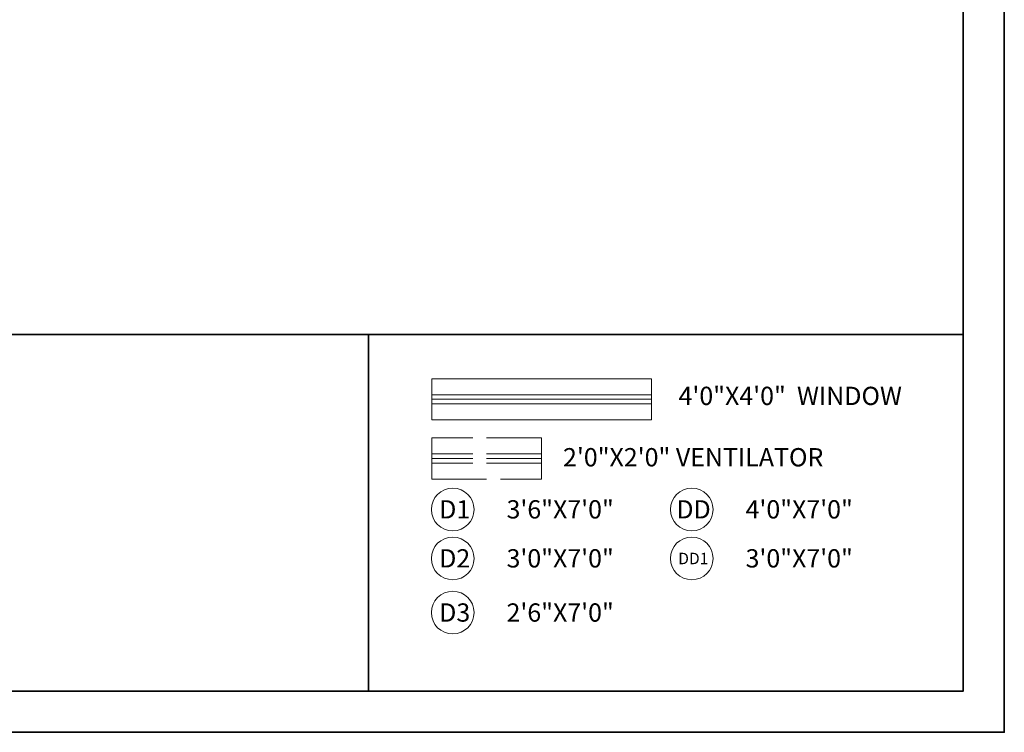
# Model space of a CAD drawing. Units: inches. Extents: x 1077 to 2505, y 1892 to 2728.
# Tile 6 of 26: x 1433 to 1648, y 1892 to 2048. Entities that reach past the tile are written whole.
import ezdxf

# ---------------------------------------------------------------- set-up
doc = ezdxf.new("R2010")
doc.units = ezdxf.units.IN
doc.linetypes.add('ACAD_ISO02W100', pattern=[15, 12, -3])
for name, color, linetype, lineweight in [('A-ANNO-LEGD', 7, 'Continuous', 13), ('A-ANNO-TTLB', 7, 'Continuous', 35), ('A-GLAZ-VENT', 6, 'ACAD_ISO02W100', 13), ('WINDOW', 160, 'Continuous', 13)]:
    doc.layers.add(name, color=color, linetype=linetype, lineweight=lineweight)
doc.styles.get("Standard").update_dxf_attribs({"font": 'arial.ttf'})

# ---------------------------------------------------------------- blocks, each defined once
blk = doc.blocks.new('WINDOW-48-EXT')
for p, q in [((0, 48), (0, 0)), ((3.5, 48), (3.5, 0)), ((4.5, 48), (4.5, 0)), ((5.5, 48), (5.5, 0)), ((9, 0), (9, 48))]:
    blk.add_line(p, q)
blk = doc.blocks.new('VENT-24')
for p, q in [((3.5, 24), (3.5, 0)), ((4.5, 24), (4.5, 0)), ((5.5, 24), (5.5, 0))]:
    blk.add_line(p, q)
blk.add_lwpolyline([(0, 0), (9, 0), (9, 24), (0, 24)], close=True)
blk = doc.blocks.new('SHEET-FRAME-RESIDENTIAL')
for p, q in [((9, 87.01), (534.52, 87.01)), ((404.52, 9), (404.52, 87.01))]:
    blk.add_line(p, q)
for points in [[(0, 830.04), (543.52, 830.04), (543.52, 0), (0, 0)], [(9, 821.04), (534.52, 821.04), (534.52, 9), (9, 9)]]:
    blk.add_lwpolyline(points, close=True)

msp = doc.modelspace()

# ---------------------------------------------------------------- linework, layer by layer
at = {"layer": 'A-ANNO-LEGD'}
for centre in [(1527.2, 1941.03), (1579.45, 1941.03), (1527.2, 1930.32), (1579.45, 1930.32), (1527.2, 1918.46)]:
    msp.add_circle(centre, 4.67, dxfattribs=at)
at = {"layer": 'WINDOW'}
for p, q in [((1522.62, 1969.62), (1522.62, 1960.62)), ((1570.62, 1969.62), (1570.62, 1960.62))]:
    msp.add_line(p, q, dxfattribs=at)

# ---------------------------------------------------------------- block references
at = {"layer": 'A-ANNO-TTLB'}
msp.add_blockref('SHEET-FRAME-RESIDENTIAL', (1104.25, 1892.27), dxfattribs=at)
at = {"layer": 'A-GLAZ-VENT', "rotation": 269.9999999999977}
msp.add_blockref('VENT-24', (1522.62, 1956.67), dxfattribs=at)
at = {"layer": 'WINDOW', "rotation": 89.99999999999969}
msp.add_blockref('WINDOW-48-EXT', (1570.62, 1960.62), dxfattribs=at)

# ---------------------------------------------------------------- texts
at = {"layer": 'A-ANNO-LEGD', "attachment_point": 1}
for s, width, insert, char_height in [('4\'0"X4\'0"  WINDOW', 55.3456, (1576.57, 1967.87), 4), ('2\'0"X2\'0" VENTILATOR', 67.3186, (1551.32, 1954.45), 4), ('D1', 8.4888, (1524.25, 1943.05), 4), ('3\'6"X7\'0"', 8.4888, (1538.97, 1943.05), 4), ('DD', 8.4888, (1576.09, 1943.05), 4), ('4\'0"X7\'0"', 8.4888, (1591.22, 1943.05), 4), ('D2', 8.4888, (1524.25, 1932.33), 4), ('3\'0"X7\'0"', 8.4888, (1538.97, 1932.33), 4), ('DD1', 8.4888, (1576.5, 1931.55), 2.5), ('3\'0"X7\'0"', 8.4888, (1591.22, 1932.33), 4), ('D3', 8.4888, (1524.25, 1920.48), 4), ('2\'6"X7\'0"', 8.4888, (1538.97, 1920.48), 4)]:
    msp.add_mtext_dynamic_manual_height_columns(s, width=width, gutter_width=12.5, heights=[0], dxfattribs=dict(at, insert=insert, char_height=char_height))

doc.saveas('drawing.dxf')
